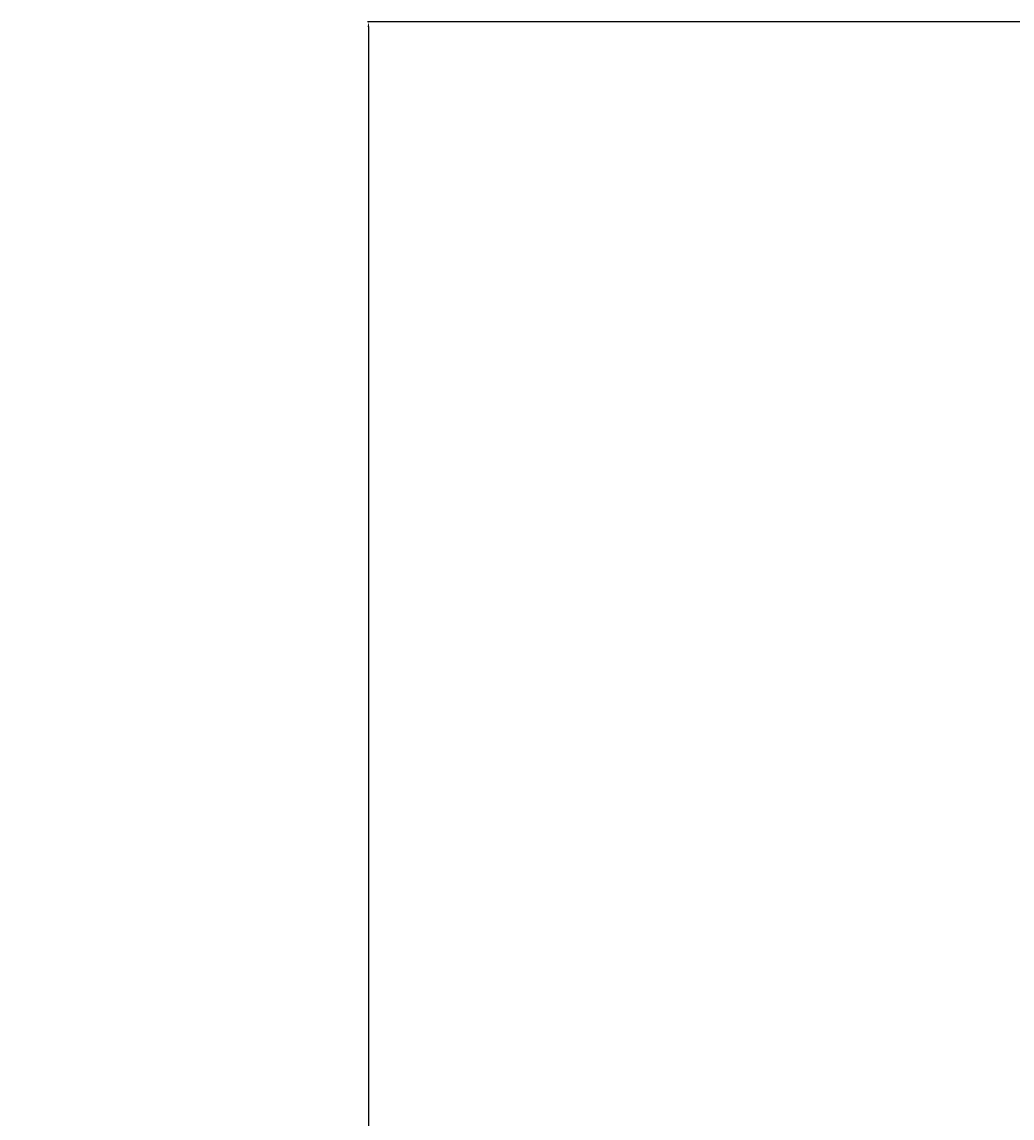
# Model space of a CAD drawing. Units: inches. Extents: x -304 to 580, y 363 to 1149.
# Tile 7 of 11: x -304 to -114, y 794 to 1005. Entities that reach past the tile are written whole.
import ezdxf

# ---------------------------------------------------------------- set-up
doc = ezdxf.new("R2010")
doc.units = ezdxf.units.IN
doc.header["$MEASUREMENT"] = 0
doc.layers.add('A-ANNO-DIMS', color=2, linetype='Continuous', lineweight=13)
doc.styles.get("Standard").update_dxf_attribs({"font": 'arial.ttf'})
doc.dimstyles.get("Standard").update_dxf_attribs({"dimtxt": 1, "dimasz": 1, "dimexe": 0.18, "dimexo": 0.0625, "dimgap": 0.09, "dimtad": 0, "dimtih": 1, "dimtoh": 1, "dimdec": 0, "dimzin": 0, "dimdsep": 46, "dimlunit": 3, "dimtxsty": 'Standard', "dimcen": 0.09, "dimadec": 0, "dimazin": 0, "dimtfac": 1, "dimtdec": 0, "dimtofl": 0, "dimtmove": 0, "dimatfit": 3, "dimfxl": 1, "dimtolj": 1, "dimtzin": 0, "dimarcsym": 0})

# ---------------------------------------------------------------- blocks, each defined once
blk = doc.blocks.new('*D1')
at = {"layer": 'A-ANNO-DIMS', "color": 0, "lineweight": -2, "transparency": 16777216}
for p, q in [((-22.63, 1004.95), (-237.62, 1004.95)), ((-237.44, 1003.95), (-237.44, 721.93)), ((-237.44, 402.95), (-237.44, 684.96)), ((-22.63, 401.95), (-237.62, 401.95))]:
    blk.add_line(p, q, dxfattribs=at)
at = {"layer": 'A-ANNO-DIMS', "color": 0, "transparency": 16777216}
for points in [[(-237.61, 1003.95), (-237.28, 1003.95), (-237.44, 1004.95)], [(-237.61, 402.95), (-237.28, 402.95), (-237.44, 401.95)]]:
    blk.add_solid(points, dxfattribs=at)
at = {"layer": 'Defpoints', "color": 0, "transparency": 16777216}
for p in [(-22.57, 1004.95), (-237.44, 401.95), (-22.57, 401.95)]:
    blk.add_point(p, dxfattribs=at)
at = {"layer": 'A-ANNO-DIMS', "color": 0, "transparency": 16777216, "insert": (-237.44, 703.45), "char_height": 1, "attachment_point": 5}
blk.add_mtext('\\A1;{\\H36x;50\'-3"}', dxfattribs=at)

msp = doc.modelspace()

# ---------------------------------------------------------------- dimensions: what is measured, and where the dimension line sits
at = {"layer": 'A-ANNO-DIMS'}
dim = msp.add_linear_dim(base=(-237.44, 401.95), p1=(-22.57, 1004.95), p2=(-22.57, 401.95), angle=90, text='{\\H36x;<>}', dimstyle='Standard', override={"dimclrd": 0, "dimclre": 0, "dimclrt": 0}, dxfattribs=at)
dim.commit()
dim.dimension.update_dxf_attribs({"geometry": '*D1', "text_midpoint": (-237.44, 703.45)})

doc.saveas('drawing.dxf')
